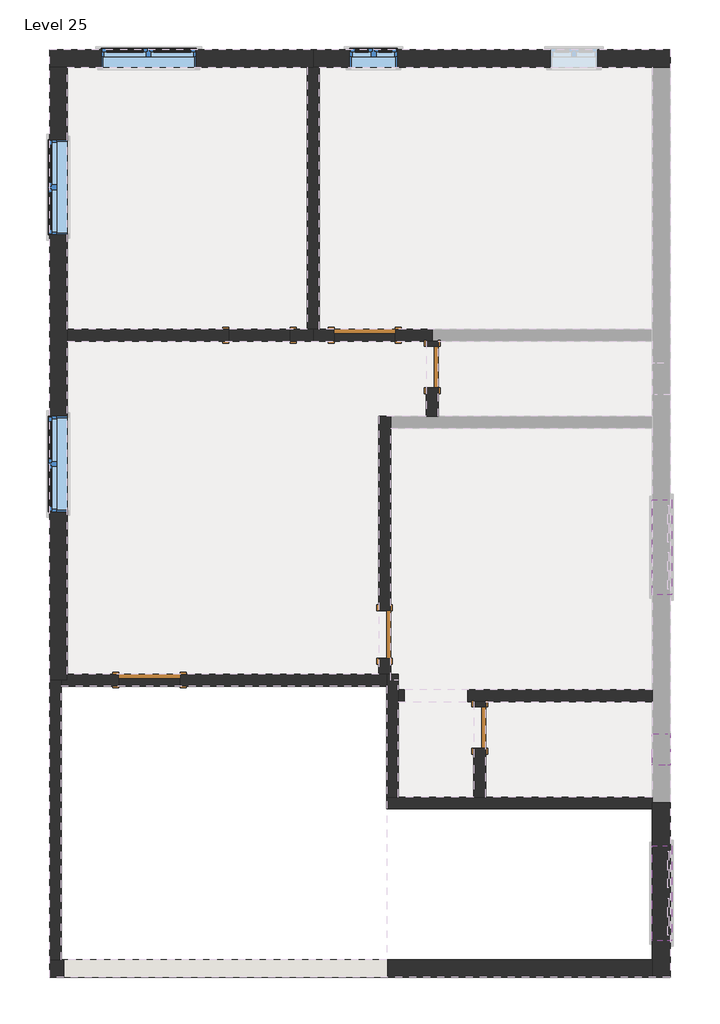
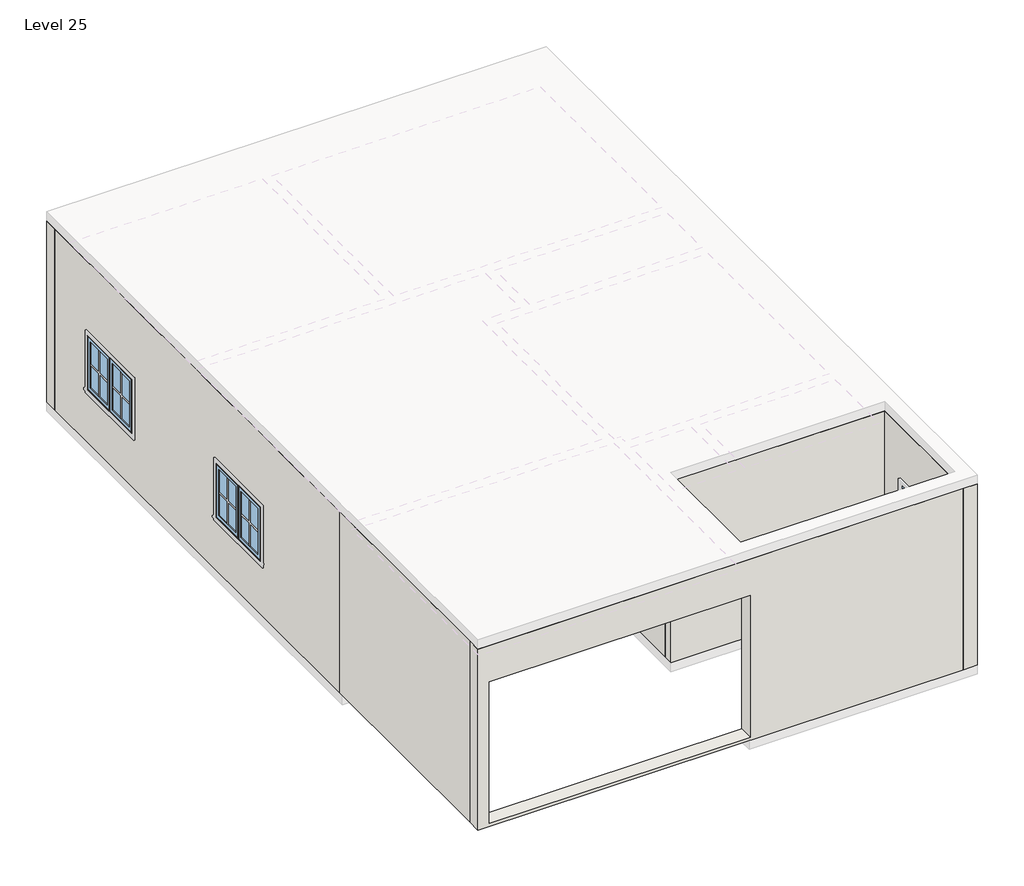
# One storey, part 1 of 2: 24 walls, 10 windows, 6 doors.
"""IFC4 building model written with IfcOpenShell, lengths in millimetres."""

from ifc_helpers import new_model, si_unit, frame, origin, place, context, project, spatial, polyline, outline, extrude, faceted_brep, transform, mapped, element, save
from components import door_2908be75, door_9ea4ff49, door_dc34e247, door_b804d09e, fixed_2_415b3208, window_casement_double_3_c417fced, window_casement_double_4_c19c33cb

model = new_model("IFC4")

# Units and contexts
model_context = context("Model", 3, world=origin())
ifc_project = project(units=[si_unit("LENGTHUNIT", "METRE", prefix="MILLI")], contexts=[model_context])

# Site, building, storey
site = spatial("IfcSite", under=ifc_project)
building = spatial("IfcBuilding", under=site)
storey = spatial("IfcBuildingStorey", under=building, Name="Level 25", Elevation=22402.8)

# Doors
placement = place(None, origin())
door_shape = door_2908be75(model_context)
element("IfcDoor", 1, ObjectType="Single-Flush : 1' 9\"", at=placement, inside=storey, context=model_context, shape_type="MappedRepresentation", body=[
    mapped(door_shape, transform((-397.3154463, -2781.5544725, 22402.8), x_axis=(0.0, 1.0, 0.0), y_axis=(-1.0, 0.0, 0.0), z_axis=(0.0, 0.0, 1.0))),
])
element("IfcDoor", 2, ObjectType="Single-Flush : 1' 9\"", at=placement, inside=storey, context=model_context, shape_type="MappedRepresentation", body=[
    mapped(door_shape, transform((-1006.9154463, 1841.2455275, 22402.8), x_axis=(0.0, 1.0, 0.0), y_axis=(-1.0, 0.0, 0.0), z_axis=(0.0, 0.0, 1.0))),
])
door_2_shape = door_9ea4ff49(model_context)
element("IfcDoor", 3, ObjectType="Single-Flush : 2'0\"", at=placement, inside=storey, context=model_context, shape_type="MappedRepresentation", body=[
    mapped(door_2_shape, transform((-1616.5154463, -1587.7544725, 22402.8), x_axis=(0.0, -1.0, 0.0), y_axis=(1.0, 0.0, 0.0), z_axis=(0.0, 0.0, 1.0))),
])
door_3_shape = door_dc34e247(model_context)
element("IfcDoor", 4, ObjectType="Single-Flush : 2'7\"", at=placement, inside=storey, context=model_context, shape_type="MappedRepresentation", body=[
    mapped(door_3_shape, transform((-4626.4154463, -2171.9544725, 22402.8), x_axis=(-1.0, 0.0, 0.0), y_axis=(0.0, -1.0, 0.0), z_axis=(0.0, 0.0, 1.0))),
])
element("IfcDoor", 5, ObjectType="Single-Flush : 2'7\"", at=placement, inside=storey, context=model_context, shape_type="MappedRepresentation", body=[
    mapped(door_3_shape, transform((-1870.5154463, 2247.6455275, 22402.8), x_axis=(-1.0, 0.0, 0.0), y_axis=(0.0, -1.0, 0.0), z_axis=(0.0, 0.0, 1.0))),
])
door_4_shape = door_b804d09e(model_context)
element("IfcDoor", 6, ObjectType="Single-Flush : 2'7\"", at=placement, inside=storey, context=model_context, shape_type="MappedRepresentation", body=[
    mapped(door_4_shape, transform((-3216.7154463, 2247.6455275, 22402.8), x_axis=(1.0, 0.0, 0.0), y_axis=(0.0, 1.0, 0.0), z_axis=(0.0, 0.0, 1.0))),
])

# Walls
element("IfcWall", 7, ObjectType="Generic - 6\"", at=placement, inside=storey, context=model_context, shape_type="Brep", body=[
    faceted_brep([(-5909.1154463, -2171.9544725, 22402.8), (-5909.1154463, -5753.3544725, 22402.8), (-5909.1154463, -5753.3544725, 25450.8), (-5909.1154463, -2171.9544725, 25450.8), (-5756.7154463, -2171.9544725, 22402.8), (-5756.7154463, -2171.9544725, 25450.8), (-5756.7154463, -2248.1544725, 25450.8), (-5756.7154463, -5753.3544725, 25450.8), (-5756.7154463, -5753.3544725, 22402.8), (-5756.7154463, -2248.1544725, 22402.8)], [[[0, 1, 2, 3]], [[4, 5, 6, 7, 8, 9]], [[1, 0, 4, 9, 8]], [[3, 2, 7, 6, 5]], [[0, 3, 5, 4]], [[2, 1, 8, 7]]]),
])
element("IfcWall", 8, ObjectType="Generic - 6\"", at=placement, inside=storey, context=model_context, shape_type="Brep", body=[
    faceted_brep([(1812.4845537, -3670.5544725, 22402.8), (-321.1154463, -3670.5544725, 22402.8), (-473.5154463, -3670.5544725, 22402.8), (-1438.7154463, -3670.5544725, 22402.8), (-1591.1154463, -3670.5544725, 22402.8), (-1591.1154463, -3670.5544725, 25450.8), (-1438.7154463, -3670.5544725, 25450.8), (-473.5154463, -3670.5544725, 25450.8), (-321.1154463, -3670.5544725, 25450.8), (1812.4845537, -3670.5544725, 25450.8), (1812.4845537, -3822.9544725, 22402.8), (1812.4845537, -3822.9544725, 25450.8), (-1591.1154463, -3822.9544725, 25450.8), (-1591.1154463, -3822.9544725, 22402.8), (1812.4845537, -3746.7544725, 22402.8), (1812.4845537, -3746.7544725, 25450.8)], [[[0, 1, 2, 3, 4, 5, 6, 7, 8, 9]], [[10, 11, 12, 13]], [[4, 3, 2, 1, 0, 14, 10, 13]], [[9, 8, 7, 6, 5, 12, 11, 15]], [[5, 4, 13, 12]], [[0, 9, 15, 11, 10, 14]]]),
])
element("IfcWall", 9, ObjectType="Generic - 6\"", at=placement, inside=storey, context=model_context, shape_type="Brep", body=[
    faceted_brep([(-1438.7154463, -3670.5544725, 22402.8), (-1438.7154463, -2451.3544725, 22402.8), (-1438.7154463, -2298.9544725, 22402.8), (-1438.7154463, -2095.7544725, 22402.8), (-1438.7154463, -2095.7544725, 25450.8), (-1438.7154463, -2298.9544725, 25450.8), (-1438.7154463, -2451.3544725, 25450.8), (-1438.7154463, -3670.5544725, 25450.8), (-1591.1154463, -3670.5544725, 22402.8), (-1591.1154463, -3670.5544725, 25450.8), (-1591.1154463, -2248.1544725, 25450.8), (-1591.1154463, -2171.9544725, 25450.8), (-1591.1154463, -2095.7544725, 25450.8), (-1591.1154463, -2095.7544725, 22402.8), (-1591.1154463, -2171.9544725, 22402.8), (-1591.1154463, -2248.1544725, 22402.8), (-1540.3154463, -2095.7544725, 22402.8), (-1540.3154463, -2095.7544725, 25450.8)], [[[0, 1, 2, 3, 4, 5, 6, 7]], [[8, 9, 10, 11, 12, 13, 14, 15]], [[3, 2, 1, 0, 8, 15, 14, 13, 16]], [[7, 6, 5, 4, 17, 12, 11, 10, 9]], [[0, 7, 9, 8]], [[4, 3, 16, 13, 12, 17]]]),
])
element("IfcWall", 10, ObjectType="Generic - 6\"", at=placement, inside=storey, context=model_context, shape_type="Brep", body=[
    faceted_brep([(-5020.1154463, -2095.7544725, 24536.4), (-5020.1154463, -2095.7544725, 22402.8), (-5680.5154463, -2095.7544725, 22402.8), (-5680.5154463, -2095.7544725, 25450.8), (-1692.7154463, -2095.7544725, 25450.8), (-1591.1154463, -2095.7544725, 25450.8), (-1591.1154463, -2095.7544725, 22402.8), (-1692.7154463, -2095.7544725, 22402.8), (-4232.7154463, -2095.7544725, 22402.8), (-4232.7154463, -2095.7544725, 24536.4), (-5756.7154463, -2248.1544725, 22402.8), (-5020.1154463, -2248.1544725, 22402.8), (-5020.1154463, -2248.1544725, 24536.4), (-4232.7154463, -2248.1544725, 24536.4), (-4232.7154463, -2248.1544725, 22402.8), (-1591.1154463, -2248.1544725, 22402.8), (-1591.1154463, -2248.1544725, 25450.8), (-5756.7154463, -2248.1544725, 25450.8), (-5756.7154463, -2171.9544725, 22402.8), (-5680.5154463, -2171.9544725, 22402.8), (-5680.5154463, -2171.9544725, 25450.8), (-5756.7154463, -2171.9544725, 25450.8)], [[[0, 1, 2, 3, 4, 5, 6, 7, 8, 9]], [[10, 11, 12, 13, 14, 15, 16, 17]], [[2, 1, 11, 10, 18, 19]], [[8, 7, 6, 15, 14]], [[5, 4, 3, 20, 21, 17, 16]], [[3, 2, 19, 20]], [[19, 18, 21, 20]], [[18, 10, 17, 21]], [[6, 5, 16, 15]], [[12, 11, 1, 0]], [[13, 12, 0, 9]], [[14, 13, 9, 8]]]),
])
element("IfcWall", 11, ObjectType="Generic - 6\"", at=placement, inside=storey, context=model_context, shape_type="Brep", body=[
    faceted_brep([(1812.4845537, -2451.3544725, 22402.8), (1812.4845537, -2451.3544725, 25450.8), (-321.1154463, -2451.3544725, 25450.8), (-473.5154463, -2451.3544725, 25450.8), (-1438.7154463, -2451.3544725, 25450.8), (-1438.7154463, -2451.3544725, 22402.8), (-1367.0206652, -2451.3544725, 22402.8), (-1367.0206652, -2451.3544725, 24841.2), (-547.4818767, -2451.3544725, 24841.2), (-547.4818767, -2451.3544725, 22402.8), (-473.5154463, -2451.3544725, 22402.8), (-321.1154463, -2451.3544725, 22402.8), (1812.4845537, -2298.9544725, 25450.8), (1812.4845537, -2298.9544725, 22402.8), (-547.4818767, -2298.9544725, 22402.8), (-547.4818767, -2298.9544725, 24841.2), (-1367.0206652, -2298.9544725, 24841.2), (-1367.0206652, -2298.9544725, 22402.8), (-1438.7154463, -2298.9544725, 22402.8), (-1438.7154463, -2298.9544725, 25450.8)], [[[0, 1, 2, 3, 4, 5, 6, 7, 8, 9, 10, 11]], [[12, 13, 14, 15, 16, 17, 18, 19]], [[5, 18, 17, 6]], [[13, 0, 11, 10, 9, 14]], [[4, 3, 2, 1, 12, 19]], [[1, 0, 13, 12]], [[5, 4, 19, 18]], [[7, 16, 15, 8]], [[16, 7, 6, 17]], [[8, 15, 14, 9]]]),
])
element("IfcWall", 12, ObjectType="Generic - 6\"", at=placement, inside=storey, context=model_context, shape_type="SweptSolid", body=[
    extrude(outline(polyline([(-2451.3544725, 22402.8), (-2514.8544725, 22402.8), (-2514.8544725, 24536.4), (-3048.2544725, 24536.4), (-3048.2544725, 22402.8), (-3670.5544725, 22402.8), (-3670.5544725, 25450.8), (-2451.3544725, 25450.8), (-2451.3544725, 22402.8)])), frame((-473.5154463, 0.0, 0.0), z_axis=(1.0, 0.0, 0.0), x_axis=(0.0, 1.0, 0.0)), (0.0, 0.0, 1.0), 152.4),
])
element("IfcWall", 13, ObjectType="Generic - 6\"", at=placement, inside=storey, context=model_context, shape_type="Brep", body=[
    faceted_brep([(-1540.3154463, -2095.7544725, 22402.8), (-1540.3154463, -1892.5544725, 22402.8), (-1540.3154463, -1892.5544725, 24536.4), (-1540.3154463, -1282.9544725, 24536.4), (-1540.3154463, -1282.9544725, 22402.8), (-1540.3154463, 1053.8455275, 22402.8), (-1540.3154463, 1206.2455275, 22402.8), (-1540.3154463, 1206.2455275, 25450.8), (-1540.3154463, 1053.8455275, 25450.8), (-1540.3154463, -2095.7544725, 25450.8), (-1692.7154463, -1892.5544725, 24536.4), (-1692.7154463, -1892.5544725, 22402.8), (-1692.7154463, -2095.7544725, 22402.8), (-1692.7154463, -2095.7544725, 25450.8), (-1692.7154463, 1206.2455275, 25450.8), (-1692.7154463, 1206.2455275, 22402.8), (-1692.7154463, -1282.9544725, 22402.8), (-1692.7154463, -1282.9544725, 24536.4), (-1591.1154463, -2095.7544725, 22402.8), (-1591.1154463, -2095.7544725, 25450.8)], [[[0, 1, 2, 3, 4, 5, 6, 7, 8, 9]], [[10, 11, 12, 13, 14, 15, 16, 17]], [[16, 15, 6, 5, 4]], [[12, 11, 1, 0, 18]], [[9, 8, 7, 14, 13, 19]], [[0, 9, 19, 13, 12, 18]], [[7, 6, 15, 14]], [[2, 1, 11, 10]], [[3, 2, 10, 17]], [[4, 3, 17, 16]]]),
])
element("IfcWall", 14, ObjectType="Generic - 6\"", at=placement, inside=storey, context=model_context, shape_type="Brep", body=[
    faceted_brep([(-930.7154463, 2107.9455275, 24536.4), (-930.7154463, 2107.9455275, 22402.8), (-930.7154463, 2171.4455275, 22402.8), (-930.7154463, 2171.4455275, 25450.8), (-930.7154463, 1206.2455275, 25450.8), (-930.7154463, 1206.2455275, 22402.8), (-930.7154463, 1574.5455275, 22402.8), (-930.7154463, 1574.5455275, 24536.4), (-1083.1154463, 2171.4455275, 22402.8), (-1083.1154463, 2107.9455275, 22402.8), (-1083.1154463, 2107.9455275, 24536.4), (-1083.1154463, 1574.5455275, 24536.4), (-1083.1154463, 1574.5455275, 22402.8), (-1083.1154463, 1206.2455275, 22402.8), (-1083.1154463, 1206.2455275, 25450.8), (-1083.1154463, 2171.4455275, 25450.8), (-1006.9154463, 2171.4455275, 22402.8), (-1006.9154463, 2171.4455275, 25450.8)], [[[0, 1, 2, 3, 4, 5, 6, 7]], [[8, 9, 10, 11, 12, 13, 14, 15]], [[6, 5, 13, 12]], [[2, 1, 9, 8, 16]], [[4, 3, 17, 15, 14]], [[5, 4, 14, 13]], [[10, 9, 1, 0]], [[11, 10, 0, 7]], [[12, 11, 7, 6]], [[3, 2, 16, 8, 15, 17]]]),
])
element("IfcWall", 15, ObjectType="Generic - 6\"", at=placement, inside=storey, context=model_context, shape_type="Brep", body=[
    faceted_brep([(-2607.1154463, 5678.2330275, 22402.8), (-2607.1154463, 2323.8455275, 22402.8), (-2607.1154463, 2323.8455275, 25450.8), (-2607.1154463, 5678.2330275, 25450.8), (-2454.7154463, 5678.2330275, 22402.8), (-2454.7154463, 5678.2330275, 25450.8), (-2454.7154463, 2323.8455275, 25450.8), (-2454.7154463, 2323.8455275, 22402.8), (-2530.9154463, 5678.2330275, 22402.8), (-2530.9154463, 2323.8455275, 22402.8), (-2530.9154463, 2323.8455275, 25450.8), (-2530.9154463, 5678.2330275, 25450.8)], [[[0, 1, 2, 3]], [[4, 5, 6, 7]], [[1, 0, 8, 4, 7, 9]], [[3, 2, 10, 6, 5, 11]], [[0, 3, 11, 5, 4, 8]], [[2, 1, 9, 7, 6, 10]]]),
])
element("IfcWall", 16, ObjectType="Generic - 6\"", at=placement, inside=storey, context=model_context, shape_type="Brep", body=[
    faceted_brep([(-2530.9154463, 2323.8455275, 22402.8), (-2607.1154463, 2323.8455275, 22402.8), (-2823.0154463, 2323.8455275, 22402.8), (-2823.0154463, 2323.8455275, 24536.4), (-3610.4154463, 2323.8455275, 24536.4), (-3610.4154463, 2323.8455275, 22402.8), (-5680.5154463, 2323.8455275, 22402.8), (-5680.5154463, 2323.8455275, 25450.8), (-2607.1154463, 2323.8455275, 25450.8), (-2530.9154463, 2323.8455275, 25450.8), (-2823.0154463, 2171.4455275, 24536.4), (-2823.0154463, 2171.4455275, 22402.8), (-2530.9154463, 2171.4455275, 22402.8), (-2530.9154463, 2171.4455275, 25450.8), (-5680.5154463, 2171.4455275, 25450.8), (-5680.5154463, 2171.4455275, 22402.8), (-3610.4154463, 2171.4455275, 22402.8), (-3610.4154463, 2171.4455275, 24536.4)], [[[0, 1, 2, 3, 4, 5, 6, 7, 8, 9]], [[10, 11, 12, 13, 14, 15, 16, 17]], [[16, 15, 6, 5]], [[12, 11, 2, 1, 0]], [[9, 8, 7, 14, 13]], [[0, 9, 13, 12]], [[7, 6, 15, 14]], [[5, 4, 17, 16]], [[4, 3, 10, 17]], [[3, 2, 11, 10]]]),
])
element("IfcWall", 17, ObjectType="Generic - 6\"", at=placement, inside=storey, context=model_context, shape_type="Brep", body=[
    faceted_brep([(-2264.2154463, 2323.8455275, 24536.4), (-2264.2154463, 2323.8455275, 22402.8), (-2454.7154463, 2323.8455275, 22402.8), (-2530.9154463, 2323.8455275, 22402.8), (-2530.9154463, 2323.8455275, 25450.8), (-2454.7154463, 2323.8455275, 25450.8), (-1006.9154463, 2323.8455275, 25450.8), (-1006.9154463, 2323.8455275, 22402.8), (-1476.8154463, 2323.8455275, 22402.8), (-1476.8154463, 2323.8455275, 24536.4), (-2530.9154463, 2171.4455275, 22402.8), (-2264.2154463, 2171.4455275, 22402.8), (-2264.2154463, 2171.4455275, 24536.4), (-1476.8154463, 2171.4455275, 24536.4), (-1476.8154463, 2171.4455275, 22402.8), (-1083.1154463, 2171.4455275, 22402.8), (-1006.9154463, 2171.4455275, 22402.8), (-1006.9154463, 2171.4455275, 25450.8), (-1083.1154463, 2171.4455275, 25450.8), (-2530.9154463, 2171.4455275, 25450.8)], [[[0, 1, 2, 3, 4, 5, 6, 7, 8, 9]], [[10, 11, 12, 13, 14, 15, 16, 17, 18, 19]], [[8, 7, 16, 15, 14]], [[3, 2, 1, 11, 10]], [[4, 3, 10, 19]], [[6, 5, 4, 19, 18, 17]], [[7, 6, 17, 16]], [[14, 13, 9, 8]], [[13, 12, 0, 9]], [[12, 11, 1, 0]]]),
])
element("IfcWall", 18, ObjectType="Generic - 6\"", at=placement, inside=storey, context=model_context, shape_type="SweptSolid", body=[
    extrude(outline(polyline([(-5680.5154463, -2095.7544725), (-1692.7154463, -2095.7544725), (-1692.7154463, -2171.9544725), (-1591.1154463, -2171.9544725), (-1591.1154463, -2248.1544725), (-5756.7154463, -2248.1544725), (-5756.7154463, -2171.9544725), (-5680.5154463, -2171.9544725), (-5680.5154463, -2095.7544725)])), frame((0.0, 0.0, 22402.8), z_axis=(0.0, 0.0, 1.0), x_axis=(1.0, 0.0, 0.0)), (0.0, 0.0, 1.0), 3048.0),
])
element("IfcWall", 19, ObjectType="Generic - 6\"", at=placement, inside=storey, context=model_context, shape_type="Brep", body=[
    faceted_brep([(-2607.1154463, 5678.2330275, 22402.8), (-2607.1154463, 2323.8455275, 22402.8), (-2607.1154463, 2323.8455275, 25450.8), (-2607.1154463, 5678.2330275, 25450.8), (-2454.7154463, 5678.2330275, 22402.8), (-2454.7154463, 5678.2330275, 25450.8), (-2454.7154463, 2323.8455275, 25450.8), (-2454.7154463, 2323.8455275, 22402.8), (-2530.9154463, 5678.2330275, 22402.8), (-2530.9154463, 2323.8455275, 22402.8), (-2530.9154463, 2323.8455275, 25450.8), (-2530.9154463, 5678.2330275, 25450.8)], [[[0, 1, 2, 3]], [[4, 5, 6, 7]], [[1, 0, 8, 4, 7, 9]], [[3, 2, 10, 6, 5, 11]], [[0, 3, 11, 5, 4, 8]], [[2, 1, 9, 7, 6, 10]]]),
])
element("IfcWall", 20, ObjectType="Generic - 6\"", at=placement, inside=storey, context=model_context, shape_type="Brep", body=[
    faceted_brep([(-2530.9154463, 2323.8455275, 22402.8), (-2607.1154463, 2323.8455275, 22402.8), (-5680.5154463, 2323.8455275, 22402.8), (-5680.5154463, 2323.8455275, 25450.8), (-2607.1154463, 2323.8455275, 25450.8), (-2530.9154463, 2323.8455275, 25450.8), (-2530.9154463, 2171.4455275, 22402.8), (-2530.9154463, 2171.4455275, 25450.8), (-5680.5154463, 2171.4455275, 25450.8), (-5680.5154463, 2171.4455275, 22402.8)], [[[0, 1, 2, 3, 4, 5]], [[6, 7, 8, 9]], [[2, 1, 0, 6, 9]], [[5, 4, 3, 8, 7]], [[0, 5, 7, 6]], [[3, 2, 9, 8]]]),
])
element("IfcWall", 21, ObjectType="Generic - 6\"", at=placement, inside=storey, context=model_context, shape_type="Brep", body=[
    faceted_brep([(-1006.9154463, 2323.8455275, 22402.8), (-2454.7154463, 2323.8455275, 22402.8), (-2530.9154463, 2323.8455275, 22402.8), (-2530.9154463, 2323.8455275, 25450.8), (-2454.7154463, 2323.8455275, 25450.8), (-1006.9154463, 2323.8455275, 25450.8), (-1006.9154463, 2171.4455275, 22402.8), (-1006.9154463, 2171.4455275, 25450.8), (-1083.1154463, 2171.4455275, 25450.8), (-2530.9154463, 2171.4455275, 25450.8), (-2530.9154463, 2171.4455275, 22402.8), (-1083.1154463, 2171.4455275, 22402.8)], [[[0, 1, 2, 3, 4, 5]], [[6, 7, 8, 9, 10, 11]], [[2, 1, 0, 6, 11, 10]], [[3, 2, 10, 9]], [[5, 4, 3, 9, 8, 7]], [[0, 5, 7, 6]]]),
])
element("IfcWall", 22, ObjectType="Generic - 9\"", at=placement, inside=storey, context=model_context, shape_type="Brep", body=[
    faceted_brep([(-5909.1154463, 5678.2330275, 22402.8), (-5680.5154463, 5678.2330275, 22402.8), (-2607.1154463, 5678.2330275, 22402.8), (-2530.9154463, 5678.2330275, 22402.8), (-2530.9154463, 5678.2330275, 25450.8), (-2607.1154463, 5678.2330275, 25450.8), (-5680.5154463, 5678.2330275, 25450.8), (-5909.1154463, 5678.2330275, 25450.8), (-4029.5154463, 5678.2330275, 24231.6), (-4029.5154463, 5678.2330275, 23317.2), (-5248.7154463, 5678.2330275, 23317.2), (-5248.7154463, 5678.2330275, 24231.6), (-5909.1154463, 5906.8330275, 22402.8), (-5909.1154463, 5906.8330275, 25450.8), (-2530.9154463, 5906.8330275, 25450.8), (-2530.9154463, 5906.8330275, 22402.8), (-4029.5154463, 5906.8330275, 24231.6), (-5248.7154463, 5906.8330275, 24231.6), (-5248.7154463, 5906.8330275, 23317.2), (-4029.5154463, 5906.8330275, 23317.2)], [[[0, 1, 2, 3, 4, 5, 6, 7], [8, 9, 10, 11]], [[12, 13, 14, 15], [16, 17, 18, 19]], [[3, 2, 1, 0, 12, 15]], [[4, 3, 15, 14]], [[7, 6, 5, 4, 14, 13]], [[0, 7, 13, 12]], [[9, 8, 16, 19]], [[10, 9, 19, 18]], [[11, 10, 18, 17]], [[8, 11, 17, 16]]]),
])
element("IfcWall", 23, ObjectType="Generic - 9\"", at=placement, inside=storey, context=model_context, shape_type="Brep", body=[
    faceted_brep([(1812.4845537, -5753.3544725, 22402.8), (-5756.7154463, -5753.3544725, 22402.8), (-5909.1154463, -5753.3544725, 22402.8), (-5909.1154463, -5753.3544725, 25450.8), (-5756.7154463, -5753.3544725, 25450.8), (1812.4845537, -5753.3544725, 25450.8), (-1576.8982041, -5753.3544725, 24841.2), (-5729.1673724, -5753.3544725, 24841.2), (-5729.1673724, -5753.3544725, 22453.6), (-1576.8982041, -5753.3544725, 22453.6), (-5909.1154463, -5981.9544725, 22402.8), (1812.4845537, -5981.9544725, 22402.8), (1812.4845537, -5981.9544725, 25450.8), (-5909.1154463, -5981.9544725, 25450.8), (-5729.1673724, -5981.9544725, 24841.2), (-1576.8982041, -5981.9544725, 24841.2), (-1576.8982041, -5981.9544725, 22453.6), (-5729.1673724, -5981.9544725, 22453.6)], [[[0, 1, 2, 3, 4, 5], [6, 7, 8, 9]], [[10, 11, 12, 13], [14, 15, 16, 17]], [[2, 1, 0, 11, 10]], [[5, 4, 3, 13, 12]], [[0, 5, 12, 11]], [[6, 15, 14, 7]], [[8, 17, 16, 9]], [[15, 6, 9, 16]], [[7, 14, 17, 8]], [[3, 2, 10, 13]]]),
])
element("IfcWall", 24, ObjectType="Generic - 9\"", at=placement, inside=storey, context=model_context, shape_type="Brep", body=[
    faceted_brep([(-5909.1154463, 5678.2330275, 22402.8), (-5909.1154463, -2171.9544725, 22402.8), (-5909.1154463, -2171.9544725, 25450.8), (-5909.1154463, 5678.2330275, 25450.8), (-5909.1154463, 4751.1330275, 24231.6), (-5909.1154463, 3531.9330275, 24231.6), (-5909.1154463, 3531.9330275, 23317.2), (-5909.1154463, 4751.1330275, 23317.2), (-5909.1154463, 1206.2455275, 24231.6), (-5909.1154463, -12.9544725, 24231.6), (-5909.1154463, -12.9544725, 23317.2), (-5909.1154463, 1206.2455275, 23317.2), (-5680.5154463, 5678.2330275, 22402.8), (-5680.5154463, 5678.2330275, 25450.8), (-5680.5154463, 2323.8455275, 25450.8), (-5680.5154463, 2171.4455275, 25450.8), (-5680.5154463, -2095.7544725, 25450.8), (-5680.5154463, -2171.9544725, 25450.8), (-5680.5154463, -2171.9544725, 22402.8), (-5680.5154463, -2095.7544725, 22402.8), (-5680.5154463, 2171.4455275, 22402.8), (-5680.5154463, 2323.8455275, 22402.8), (-5680.5154463, 4751.1330275, 24231.6), (-5680.5154463, 4751.1330275, 23317.2), (-5680.5154463, 3531.9330275, 23317.2), (-5680.5154463, 3531.9330275, 24231.6), (-5680.5154463, 1206.2455275, 24231.6), (-5680.5154463, 1206.2455275, 23317.2), (-5680.5154463, -12.9544725, 23317.2), (-5680.5154463, -12.9544725, 24231.6), (-5756.7154463, -2171.9544725, 22402.8), (-5756.7154463, -2171.9544725, 25450.8)], [[[0, 1, 2, 3], [4, 5, 6, 7], [8, 9, 10, 11]], [[12, 13, 14, 15, 16, 17, 18, 19, 20, 21], [22, 23, 24, 25], [26, 27, 28, 29]], [[1, 0, 12, 21, 20, 19, 18, 30]], [[2, 1, 30, 18, 17, 31]], [[3, 2, 31, 17, 16, 15, 14, 13]], [[0, 3, 13, 12]], [[23, 22, 4, 7]], [[24, 23, 7, 6]], [[25, 24, 6, 5]], [[22, 25, 5, 4]], [[27, 26, 8, 11]], [[28, 27, 11, 10]], [[29, 28, 10, 9]], [[26, 29, 9, 8]]]),
])
element("IfcWall", 25, ObjectType="Generic - 9\"", at=placement, inside=storey, context=model_context, shape_type="Brep", body=[
    faceted_brep([(-2530.9154463, 5678.2330275, 22402.8), (-2454.7154463, 5678.2330275, 22402.8), (1812.4845537, 5678.2330275, 22402.8), (2041.0845537, 5678.2330275, 22402.8), (2041.0845537, 5678.2330275, 25450.8), (1812.4845537, 5678.2330275, 25450.8), (-2454.7154463, 5678.2330275, 25450.8), (-2530.9154463, 5678.2330275, 25450.8), (-1451.4154463, 5678.2330275, 24231.6), (-1451.4154463, 5678.2330275, 23317.2), (-2061.0154463, 5678.2330275, 23317.2), (-2061.0154463, 5678.2330275, 24231.6), (1113.9845537, 5678.2330275, 24231.6), (1113.9845537, 5678.2330275, 23317.2), (504.3845537, 5678.2330275, 23317.2), (504.3845537, 5678.2330275, 24231.6), (-2530.9154463, 5906.8330275, 22402.8), (-2530.9154463, 5906.8330275, 25450.8), (2041.0845537, 5906.8330275, 25450.8), (2041.0845537, 5906.8330275, 22402.8), (-1451.4154463, 5906.8330275, 24231.6), (-2061.0154463, 5906.8330275, 24231.6), (-2061.0154463, 5906.8330275, 23317.2), (-1451.4154463, 5906.8330275, 23317.2), (1113.9845537, 5906.8330275, 24231.6), (504.3845537, 5906.8330275, 24231.6), (504.3845537, 5906.8330275, 23317.2), (1113.9845537, 5906.8330275, 23317.2)], [[[0, 1, 2, 3, 4, 5, 6, 7], [8, 9, 10, 11], [12, 13, 14, 15]], [[16, 17, 18, 19], [20, 21, 22, 23], [24, 25, 26, 27]], [[3, 2, 1, 0, 16, 19]], [[7, 6, 5, 4, 18, 17]], [[0, 7, 17, 16]], [[4, 3, 19, 18]], [[8, 11, 21, 20]], [[11, 10, 22, 21]], [[10, 9, 23, 22]], [[9, 8, 20, 23]], [[12, 15, 25, 24]], [[15, 14, 26, 25]], [[14, 13, 27, 26]], [[13, 12, 24, 27]]]),
])
element("IfcWall", 26, ObjectType="Generic - 9\"", at=placement, inside=storey, context=model_context, shape_type="Brep", body=[
    faceted_brep([(1812.4845537, -3746.7544725, 22402.8), (1812.4845537, -3822.9544725, 22402.8), (1812.4845537, -5753.3544725, 22402.8), (1812.4845537, -5981.9544725, 22402.8), (1812.4845537, -5981.9544725, 25450.8), (1812.4845537, -5753.3544725, 25450.8), (1812.4845537, -3822.9544725, 25450.8), (1812.4845537, -3746.7544725, 25450.8), (1812.4845537, -5512.0544725, 24536.4), (1812.4845537, -5512.0544725, 23622.0), (1812.4845537, -4292.8544725, 23622.0), (1812.4845537, -4292.8544725, 24536.4), (2041.0845537, -3746.7544725, 22402.8), (2041.0845537, -3746.7544725, 25450.8), (2041.0845537, -5981.9544725, 25450.8), (2041.0845537, -5981.9544725, 22402.8), (2041.0845537, -5512.0544725, 24536.4), (2041.0845537, -4292.8544725, 24536.4), (2041.0845537, -4292.8544725, 23622.0), (2041.0845537, -5512.0544725, 23622.0)], [[[0, 1, 2, 3, 4, 5, 6, 7], [8, 9, 10, 11]], [[12, 13, 14, 15], [16, 17, 18, 19]], [[3, 2, 1, 0, 12, 15]], [[7, 6, 5, 4, 14, 13]], [[0, 7, 13, 12]], [[4, 3, 15, 14]], [[8, 11, 17, 16]], [[11, 10, 18, 17]], [[10, 9, 19, 18]], [[9, 8, 16, 19]]]),
])
element("IfcWall", 27, ObjectType="Generic - 9\"", at=placement, inside=storey, context=model_context, shape_type="SweptSolid", body=[
    extrude(outline(polyline([(22402.8, -5680.5154463), (22402.8, -2607.1154463), (25450.8, -2607.1154463), (25450.8, -5680.5154463), (22402.8, -5680.5154463)]), holes=[polyline([(24231.6, -4029.5154463), (23317.2, -4029.5154463), (23317.2, -5248.7154463), (24231.6, -5248.7154463), (24231.6, -4029.5154463)])]), frame((0.0, 5678.2330275, 0.0), z_axis=(0.0, 1.0, 0.0), x_axis=(0.0, 0.0, 1.0)), (0.0, 0.0, 1.0), 228.6),
])
element("IfcWall", 28, ObjectType="Generic - 9\"", at=placement, inside=storey, context=model_context, shape_type="Brep", body=[
    faceted_brep([(1812.4845537, -5753.3544725, 22402.8), (-5756.7154463, -5753.3544725, 22402.8), (-5909.1154463, -5753.3544725, 22402.8), (-5909.1154463, -5753.3544725, 25450.8), (-5756.7154463, -5753.3544725, 25450.8), (1812.4845537, -5753.3544725, 25450.8), (-1576.8982041, -5753.3544725, 24841.2), (-5729.1673724, -5753.3544725, 24841.2), (-5729.1673724, -5753.3544725, 22453.6), (-1576.8982041, -5753.3544725, 22453.6), (-5909.1154463, -5981.9544725, 22402.8), (1812.4845537, -5981.9544725, 22402.8), (1812.4845537, -5981.9544725, 25450.8), (-5909.1154463, -5981.9544725, 25450.8), (-5729.1673724, -5981.9544725, 24841.2), (-1576.8982041, -5981.9544725, 24841.2), (-1576.8982041, -5981.9544725, 22453.6), (-5729.1673724, -5981.9544725, 22453.6)], [[[0, 1, 2, 3, 4, 5], [6, 7, 8, 9]], [[10, 11, 12, 13], [14, 15, 16, 17]], [[2, 1, 0, 11, 10]], [[5, 4, 3, 13, 12]], [[6, 15, 14, 7]], [[8, 17, 16, 9]], [[15, 6, 9, 16]], [[7, 14, 17, 8]], [[3, 2, 10, 13]], [[0, 5, 12, 11]]]),
])
element("IfcWall", 29, ObjectType="Generic - 9\"", at=placement, inside=storey, context=model_context, shape_type="SweptSolid", body=[
    extrude(outline(polyline([(22402.8, -2454.7154463), (22402.8, 1812.4845537), (25450.8, 1812.4845537), (25450.8, -2454.7154463), (22402.8, -2454.7154463)]), holes=[polyline([(24231.6, -1451.4154463), (23317.2, -1451.4154463), (23317.2, -2061.0154463), (24231.6, -2061.0154463), (24231.6, -1451.4154463)]), polyline([(24231.6, 1113.9845537), (23317.2, 1113.9845537), (23317.2, 504.3845537), (24231.6, 504.3845537), (24231.6, 1113.9845537)])]), frame((0.0, 5678.2330275, 0.0), z_axis=(0.0, 1.0, 0.0), x_axis=(0.0, 0.0, 1.0)), (0.0, 0.0, 1.0), 228.6),
])
element("IfcWall", 30, ObjectType="Generic - 9\"", at=placement, inside=storey, context=model_context, shape_type="SweptSolid", body=[
    extrude(outline(polyline([(-3822.9544725, 22402.8), (-5753.3544725, 22402.8), (-5753.3544725, 25450.8), (-3822.9544725, 25450.8), (-3822.9544725, 22402.8)]), holes=[polyline([(-5512.0544725, 24536.4), (-5512.0544725, 23622.0), (-4292.8544725, 23622.0), (-4292.8544725, 24536.4), (-5512.0544725, 24536.4)])]), frame((1812.4845537, 0.0, 0.0), z_axis=(1.0, 0.0, 0.0), x_axis=(0.0, 1.0, 0.0)), (0.0, 0.0, 1.0), 228.6),
])

# Windows
fixed_2_shape = fixed_2_415b3208(model_context)
element("IfcWindow", 31, ObjectType="Fixed : 2'", at=placement, inside=storey, context=model_context, shape_type="MappedRepresentation", body=[
    mapped(fixed_2_shape, transform((1926.7845537, -3099.0544725, 23926.8), x_axis=(0.0, -1.0, 0.0), y_axis=(1.0, 0.0, 0.0), z_axis=(0.0, 0.0, 1.0))),
])
window_casement_double_3_shape = window_casement_double_3_c417fced(model_context)
element("IfcWindow", 32, ObjectType="Window-Casement-Double : 3'", at=placement, inside=storey, context=model_context, shape_type="MappedRepresentation", body=[
    mapped(window_casement_double_3_shape, transform((-1756.2154463, 5792.5330275, 22402.8), x_axis=(1.0, 0.0, 0.0), y_axis=(0.0, 1.0, 0.0), z_axis=(0.0, 0.0, 1.0))),
])
element("IfcWindow", 33, ObjectType="Window-Casement-Double : 3'", at=placement, inside=storey, context=model_context, shape_type="MappedRepresentation", body=[
    mapped(window_casement_double_3_shape, transform((-1756.2154463, 5792.5330275, 22402.8), x_axis=(1.0, 0.0, 0.0), y_axis=(0.0, 1.0, 0.0), z_axis=(0.0, 0.0, 1.0))),
])
window_casement_double_4_shape = window_casement_double_4_c19c33cb(model_context)
element("IfcWindow", 34, ObjectType="Window-Casement-Double : 4'", at=placement, inside=storey, context=model_context, shape_type="MappedRepresentation", body=[
    mapped(window_casement_double_4_shape, transform((-4639.1154463, 5792.5330275, 22402.8), x_axis=(1.0, 0.0, 0.0), y_axis=(0.0, 1.0, 0.0), z_axis=(0.0, 0.0, 1.0))),
])
element("IfcWindow", 35, ObjectType="Window-Casement-Double : 4'", at=placement, inside=storey, context=model_context, shape_type="MappedRepresentation", body=[
    mapped(window_casement_double_4_shape, transform((-5794.8154463, 4141.5330275, 22402.8), x_axis=(0.0, 1.0, 0.0), y_axis=(-1.0, 0.0, 0.0), z_axis=(0.0, 0.0, 1.0))),
])
element("IfcWindow", 36, ObjectType="Window-Casement-Double : 4'", at=placement, inside=storey, context=model_context, shape_type="MappedRepresentation", body=[
    mapped(window_casement_double_4_shape, transform((-5794.8154463, 596.6455275, 22402.8), x_axis=(0.0, 1.0, 0.0), y_axis=(-1.0, 0.0, 0.0), z_axis=(0.0, 0.0, 1.0))),
])
element("IfcWindow", 37, ObjectType="Window-Casement-Double : 4'", at=placement, inside=storey, context=model_context, shape_type="MappedRepresentation", body=[
    mapped(window_casement_double_4_shape, transform((1926.7845537, -470.1544725, 22707.6), x_axis=(0.0, -1.0, 0.0), y_axis=(1.0, 0.0, 0.0), z_axis=(0.0, 0.0, 1.0))),
])
element("IfcWindow", 38, ObjectType="Window-Casement-Double : 4'", at=placement, inside=storey, context=model_context, shape_type="MappedRepresentation", body=[
    mapped(window_casement_double_4_shape, transform((1926.7845537, -4902.4544725, 22707.6), x_axis=(0.0, -1.0, 0.0), y_axis=(1.0, 0.0, 0.0), z_axis=(0.0, 0.0, 1.0))),
])
element("IfcWindow", 39, ObjectType="Window-Casement-Double : 4'", at=placement, inside=storey, context=model_context, shape_type="MappedRepresentation", body=[
    mapped(window_casement_double_4_shape, transform((-4639.1154463, 5792.5330275, 22402.8), x_axis=(1.0, 0.0, 0.0), y_axis=(0.0, 1.0, 0.0), z_axis=(0.0, 0.0, 1.0))),
])
element("IfcWindow", 40, ObjectType="Window-Casement-Double : 4'", at=placement, inside=storey, context=model_context, shape_type="MappedRepresentation", body=[
    mapped(window_casement_double_4_shape, transform((1926.7845537, -4902.4544725, 22707.6), x_axis=(0.0, -1.0, 0.0), y_axis=(1.0, 0.0, 0.0), z_axis=(0.0, 0.0, 1.0))),
])

save(model, "model.ifc")

# Revit data of these elements
# Type "Single-Flush : 1' 9\""
#   Type Mark = "10"
#   Construction Type Id = "MDOOR"
#   Assembly Code = "C1020"
#   Analytic Construction = "Metal"
#   Thickness = 0' - 2"
#   Heat Transfer Coefficient (U) = 0.651978 BTU/(h·ft²·°F)
#   Height = 7' - 0"
#   Trim Projection Ext = 0' - 1"
#   Trim Projection Int = 0' - 1"
#   Trim Width = 0' - 3"
#   Width = 1' - 9"
#   Define Thermal Properties by = 1
#   Door Material = Door - Panel
#   Frame Material = Door - Frame
#   Visual Light Transmittance = 0
#   Solar Heat Gain Coefficient = 0
#   Function = (empty or 0)
#   Wall Closure = (empty or 0)
# Type "Single-Flush : 2'0\""
#   Type Mark = "9"
#   Construction Type Id = "MDOOR"
#   Assembly Code = "C1020"
#   Analytic Construction = "Metal"
#   Thickness = 0' - 2"
#   Heat Transfer Coefficient (U) = 0.651978 BTU/(h·ft²·°F)
#   Height = 7' - 0"
#   Trim Projection Ext = 0' - 1"
#   Trim Projection Int = 0' - 1"
#   Trim Width = 0' - 3"
#   Width = 2' - 0"
#   Define Thermal Properties by = 1
#   Door Material = Door - Panel
#   Frame Material = Door - Frame
#   Visual Light Transmittance = 0
#   Solar Heat Gain Coefficient = 0
#   Function = (empty or 0)
#   Wall Closure = (empty or 0)
# Type "Single-Flush : 2'7\""
#   Type Mark = "8"
#   Construction Type Id = "MDOOR"
#   Assembly Code = "C1020"
#   Analytic Construction = "Metal"
#   Thickness = 0' - 2"
#   Heat Transfer Coefficient (U) = 0.651978 BTU/(h·ft²·°F)
#   Height = 7' - 0"
#   Trim Projection Ext = 0' - 1"
#   Trim Projection Int = 0' - 1"
#   Trim Width = 0' - 3"
#   Width = 2' - 7"
#   Define Thermal Properties by = 1
#   Door Material = Door - Panel
#   Frame Material = Door - Frame
#   Visual Light Transmittance = 0
#   Solar Heat Gain Coefficient = 0
#   Function = (empty or 0)
#   Wall Closure = (empty or 0)
# Type "Generic - 6\""
#   Assembly Code = "B2010"
#   Layers, outside or top first: 0' - 6" no material (function 1)
# Type "Generic - 9\""
#   Assembly Code = "B2010"
#   Layers, outside or top first: 0' - 9" no material (function 1)
# Type "Fixed : 2'"
#   Type Mark = "20"
#   Construction Type Id = "GSP4R"
#   Assembly Code = "B2020100"
#   Analytic Construction = "1/8 in Pilkington single glazing"
#   Visual Light Transmittance = 0.9
#   Solar Heat Gain Coefficient = 0.78
#   Heat Transfer Coefficient (U) = 0.6496 BTU/(h·ft²·°F)
#   Height = 2' - 0"
#   Default Sill Height = 1' - 0"
#   Width = 1' - 4"
#   Window Inset = 0' - 0 3/4"
#   Define Thermal Properties by = 1
#   Glass Pane Material = Glass
#   Sash Material = Sash
#   Wall Closure = (empty or 0)
# Type "Window-Casement-Double : 3'"
#   Type Mark = "19"
#   Fire Rating = "0.5h"
#   Assembly Code = "B2020100"
#   Analytic Construction = "Double glazing - domestic"
#   Frame Extension [instance default] = 0' - 0 1/4"
#   Window Inset [instance default] = 0' - 0"
#   Wall Thickness [instance default] = 0' - 6"
#   Interior Wall Closure [instance default] = 0' - 2 1/4"
#   Half Width = 1' - 0"
#   Visual Light Transmittance = 0.81
#   Thermal Resistance (R) = 1.8146 (h·ft²·°F)/BTU
#   Solar Heat Gain Coefficient = 0.76
#   Rough Width = 2' - 0 1/2"
#   Rough Height = 3' - 0 1/2"
#   Height = 3' - 0"
#   Heat Transfer Coefficient (U) = 0.5511 BTU/(h·ft²·°F)
#   Exterior Wall Closure [instance default] = 0' - 1 1/4"
#   Extension Jamb [instance default] = 0' - 2 1/4"
#   Default Sill Height = 3' - 0"
#   Width = 2' - 0"
#   Muntin Visibility = yes
#   Interior Trim Visibility [instance default] = yes
#   Exterior Trim Visibility [instance default] = yes
#   Extension Jamb Visibility [instance default] = yes
#   Interior Trim Material = Wood - Stained
#   Muntin Pattern = Muntin Pattern_2x2 : Muntin Pattern_2x2
#   Interior Trim = Trim-Window-Interior-Flat : Picture Frame
#   Interior Frame Material = Wood - Stained
#   Glass Panel Material = Glass
#   Exterior Trim Material = Clad - White
#   Exterior Trim = Trim-Window-Exterior-Flat : with Sill
#   Exterior Frame Material = Clad - White
#   Wall Closure = (empty or 0)
# Type "Window-Casement-Double : 4'"
#   Type Mark = "18"
#   Fire Rating = "0.5h"
#   Assembly Code = "B2020100"
#   Analytic Construction = "Double glazing - domestic"
#   Frame Extension [instance default] = 0' - 0 1/4"
#   Window Inset [instance default] = 0' - 0"
#   Wall Thickness [instance default] = 0' - 6"
#   Interior Wall Closure [instance default] = 0' - 2 1/4"
#   Half Width = 2' - 0"
#   Visual Light Transmittance = 0.81
#   Thermal Resistance (R) = 1.8146 (h·ft²·°F)/BTU
#   Solar Heat Gain Coefficient = 0.76
#   Rough Width = 4' - 0 1/2"
#   Rough Height = 3' - 0 1/2"
#   Height = 3' - 0"
#   Heat Transfer Coefficient (U) = 0.5511 BTU/(h·ft²·°F)
#   Exterior Wall Closure [instance default] = 0' - 1 1/4"
#   Extension Jamb [instance default] = 0' - 2 1/4"
#   Default Sill Height = 3' - 0"
#   Width = 4' - 0"
#   Muntin Visibility = yes
#   Interior Trim Visibility [instance default] = yes
#   Exterior Trim Visibility [instance default] = yes
#   Extension Jamb Visibility [instance default] = yes
#   Interior Trim Material = Wood - Stained
#   Muntin Pattern = Muntin Pattern_2x2 : Muntin Pattern_2x2
#   Interior Trim = Trim-Window-Interior-Flat : Picture Frame
#   Interior Frame Material = Wood - Stained
#   Glass Panel Material = Glass
#   Exterior Trim Material = Clad - White
#   Exterior Trim = Trim-Window-Exterior-Flat : with Sill
#   Exterior Frame Material = Clad - White
#   Wall Closure = (empty or 0)
# Elements 1, 2 (IfcDoor, "Single-Flush : 1' 9\"")
#   Phase Created = New Construction
#   Materials on its faces: "Door - Frame", "Door - Panel"
# Element 3 (IfcDoor, "Single-Flush : 2'0\"")
#   Phase Created = New Construction
#   Materials on its faces: "Door - Frame", "Door - Panel"
# Elements 4, 5, 6 (IfcDoor, "Single-Flush : 2'7\"")
#   Phase Created = New Construction
#   Materials on its faces: "Door - Frame", "Door - Panel"
# Element 7 (IfcWall, "Generic - 6\"")
#   Top Offset = 0' - 0"
#   Base Offset = 0' - 0"
#   Unconnected Height = 10' - 0"
#   wall height = 10' - 0"
#   Phase Created = New Construction
#   Base Constraint = Level 25
#   Materials on its faces: "Default Wall", "WALL PAINT 4"
# Element 8 (IfcWall, "Generic - 6\"")
#   Top Offset = 0' - 0"
#   Base Offset = 0' - 0"
#   Unconnected Height = 10' - 0"
#   wall height = 10' - 0"
#   Phase Created = New Construction
#   Base Constraint = Level 25
#   Materials on its faces: "Default Wall", "MARBLE", "WALL PAINT 5"
# Element 9 (IfcWall, "Generic - 6\"")
#   Top Offset = 0' - 0"
#   Base Offset = 0' - 0"
#   Unconnected Height = 10' - 0"
#   wall height = 10' - 0"
#   Phase Created = New Construction
#   Base Constraint = Level 25
#   Materials on its faces: "Default Wall", "WALL PAINT 4", "MARBLE"
# Elements 10, 18 (IfcWall, "Generic - 6\"")
#   Top Offset = 0' - 0"
#   Base Offset = 0' - 0"
#   Unconnected Height = 10' - 0"
#   wall height = 10' - 0"
#   Phase Created = New Construction
#   Base Constraint = Level 25
#   Materials on its faces: "Default Wall", "WALL PAINT 2", "MARBLE"
# Element 11 (IfcWall, "Generic - 6\"")
#   Top Offset = 0' - 0"
#   Base Offset = 0' - 0"
#   Unconnected Height = 10' - 0"
#   wall height = 10' - 0"
#   Phase Created = New Construction
#   Base Constraint = Level 25
#   Materials on its faces: "Default Wall", "WALL PAINT 4", "WALL PAINT 5"
# Element 12 (IfcWall, "Generic - 6\"")
#   Top Offset = 0' - 0"
#   Base Offset = 0' - 0"
#   Unconnected Height = 10' - 0"
#   wall height = 10' - 0"
#   Phase Created = New Construction
#   Base Constraint = Level 25
#   Materials on its faces: "Default Wall", "WALL PAINT 5"
# Element 13 (IfcWall, "Generic - 6\"")
#   Top Offset = 0' - 0"
#   Base Offset = 0' - 0"
#   Unconnected Height = 10' - 0"
#   wall height = 10' - 0"
#   Phase Created = New Construction
#   Base Constraint = Level 25
#   Materials on its faces: "Default Wall", "WALL PAINT 4", "WALL PAINT 2", "WALL PAINT 5"
# Element 14 (IfcWall, "Generic - 6\"")
#   Top Offset = 0' - 0"
#   Base Offset = 0' - 0"
#   Unconnected Height = 10' - 0"
#   wall height = 10' - 0"
#   Phase Created = New Construction
#   Base Constraint = Level 25
#   Materials on its faces: "Default Wall", "WALL PAINT 5", "WALL PAINT 2"
# Elements 15, 19 (IfcWall, "Generic - 6\"")
#   Top Offset = 0' - 0"
#   Base Offset = 0' - 0"
#   Unconnected Height = 10' - 0"
#   wall height = 10' - 0"
#   Phase Created = New Construction
#   Base Constraint = Level 25
#   Materials on its faces: "Default Wall", "WALL PAINT 1", "WALL PAINT 3"
# Elements 16, 20 (IfcWall, "Generic - 6\"")
#   Top Offset = 0' - 0"
#   Base Offset = 0' - 0"
#   Unconnected Height = 10' - 0"
#   wall height = 10' - 0"
#   Phase Created = New Construction
#   Base Constraint = Level 25
#   Materials on its faces: "Default Wall", "WALL PAINT 1", "WALL PAINT 2"
# Elements 17, 21 (IfcWall, "Generic - 6\"")
#   Top Offset = 0' - 0"
#   Base Offset = 0' - 0"
#   Unconnected Height = 10' - 0"
#   wall height = 10' - 0"
#   Phase Created = New Construction
#   Base Constraint = Level 25
#   Materials on its faces: "Default Wall", "WALL PAINT 3", "WALL PAINT 2"
# Elements 22, 27 (IfcWall, "Generic - 9\"")
#   Top Offset = 0' - 0"
#   Base Offset = 0' - 0"
#   Unconnected Height = 10' - 0"
#   wall height = 10' - 0"
#   Phase Created = New Construction
#   Base Constraint = Level 25
#   Materials on its faces: "Default Wall", "WALL PAINT 1"
# Elements 23, 26, 28, 30 (IfcWall, "Generic - 9\"")
#   Top Offset = 0' - 0"
#   Base Offset = 0' - 0"
#   Unconnected Height = 10' - 0"
#   wall height = 10' - 0"
#   Phase Created = New Construction
#   Base Constraint = Level 25
#   Materials on its faces: "Default Wall", "WALL PAINT 4"
# Element 24 (IfcWall, "Generic - 9\"")
#   Top Offset = 0' - 0"
#   Base Offset = 0' - 0"
#   Unconnected Height = 10' - 0"
#   wall height = 10' - 0"
#   Phase Created = New Construction
#   Base Constraint = Level 25
#   Materials on its faces: "Default Wall"
# Elements 25, 29 (IfcWall, "Generic - 9\"")
#   Top Offset = 0' - 0"
#   Base Offset = 0' - 0"
#   Unconnected Height = 10' - 0"
#   wall height = 10' - 0"
#   Phase Created = New Construction
#   Base Constraint = Level 25
#   Materials on its faces: "Default Wall", "WALL PAINT 3"
# Element 31 (IfcWindow, "Fixed : 2'")
#   Mark = "112"
#   Phase Created = New Construction
#   Materials on its faces: "Sash", "Glass"
# Element 32 (IfcWindow, "Window-Casement-Double : 3'")
#   Mark = "110"
#   Window Inset = 0' - 0"
#   Interior Wall Closure = 0' - 2 1/4"
#   Frame Extension = 0' - 0 1/4"
#   Exterior Wall Closure = 0' - 1 1/4"
#   Interior Trim Visibility = yes
#   Exterior Trim Visibility = yes
#   Phase Created = New Construction
#   Materials on its faces: "Wood - Stained", "Glass", "Clad - White"
# Element 33 (IfcWindow, "Window-Casement-Double : 3'")
#   Mark = "116"
#   Window Inset = 0' - 0"
#   Interior Wall Closure = 0' - 2 1/4"
#   Frame Extension = 0' - 0 1/4"
#   Exterior Wall Closure = 0' - 1 1/4"
#   Interior Trim Visibility = yes
#   Exterior Trim Visibility = yes
#   Phase Created = New Construction
#   Materials on its faces: "Wood - Stained", "Glass", "Clad - White"
# Element 34 (IfcWindow, "Window-Casement-Double : 4'")
#   Mark = "105"
#   Window Inset = 0' - 0"
#   Interior Wall Closure = 0' - 2 1/4"
#   Frame Extension = 0' - 0 1/4"
#   Exterior Wall Closure = 0' - 1 1/4"
#   Interior Trim Visibility = yes
#   Exterior Trim Visibility = yes
#   Phase Created = New Construction
#   Materials on its faces: "Wood - Stained", "Glass", "Clad - White"
# Element 35 (IfcWindow, "Window-Casement-Double : 4'")
#   Mark = "106"
#   Window Inset = 0' - 0"
#   Interior Wall Closure = 0' - 2 1/4"
#   Frame Extension = 0' - 0 1/4"
#   Exterior Wall Closure = 0' - 1 1/4"
#   Interior Trim Visibility = yes
#   Exterior Trim Visibility = yes
#   Phase Created = New Construction
#   Materials on its faces: "Wood - Stained", "Glass", "Clad - White"
# Element 36 (IfcWindow, "Window-Casement-Double : 4'")
#   Mark = "107"
#   Window Inset = 0' - 0"
#   Interior Wall Closure = 0' - 2 1/4"
#   Frame Extension = 0' - 0 1/4"
#   Exterior Wall Closure = 0' - 1 1/4"
#   Interior Trim Visibility = yes
#   Exterior Trim Visibility = yes
#   Phase Created = New Construction
#   Materials on its faces: "Wood - Stained", "Glass", "Clad - White"
# Element 37 (IfcWindow, "Window-Casement-Double : 4'")
#   Mark = "108"
#   Window Inset = 0' - 0"
#   Interior Wall Closure = 0' - 2 1/4"
#   Frame Extension = 0' - 0 1/4"
#   Exterior Wall Closure = 0' - 1 1/4"
#   Interior Trim Visibility = yes
#   Exterior Trim Visibility = yes
#   Phase Created = New Construction
#   Materials on its faces: "Wood - Stained", "Glass", "Clad - White"
# Element 38 (IfcWindow, "Window-Casement-Double : 4'")
#   Mark = "109"
#   Window Inset = 0' - 0"
#   Interior Wall Closure = 0' - 2 1/4"
#   Frame Extension = 0' - 0 1/4"
#   Exterior Wall Closure = 0' - 1 1/4"
#   Interior Trim Visibility = yes
#   Exterior Trim Visibility = yes
#   Phase Created = New Construction
#   Materials on its faces: "Wood - Stained", "Glass", "Clad - White"
# Element 39 (IfcWindow, "Window-Casement-Double : 4'")
#   Mark = "114"
#   Window Inset = 0' - 0"
#   Interior Wall Closure = 0' - 2 1/4"
#   Frame Extension = 0' - 0 1/4"
#   Exterior Wall Closure = 0' - 1 1/4"
#   Interior Trim Visibility = yes
#   Exterior Trim Visibility = yes
#   Phase Created = New Construction
#   Materials on its faces: "Wood - Stained", "Glass", "Clad - White"
# Element 40 (IfcWindow, "Window-Casement-Double : 4'")
#   Mark = "115"
#   Window Inset = 0' - 0"
#   Interior Wall Closure = 0' - 2 1/4"
#   Frame Extension = 0' - 0 1/4"
#   Exterior Wall Closure = 0' - 1 1/4"
#   Interior Trim Visibility = yes
#   Exterior Trim Visibility = yes
#   Phase Created = New Construction
#   Materials on its faces: "Wood - Stained", "Glass", "Clad - White"
# Materials
#   "Door - Panel": class "Wood", colour RGB 210 159 95, transparency 0, Cost = 0
#   "Door - Frame": colour RGB 118 70 51, transparency 0, Cost = 0
#   "Glass": class "Glass", colour RGB 0 128 192, transparency 0.75, Description = "Soda Lime Glass", Cost = 0
#   "Sash": class "Wood", colour RGB 224 178 126, transparency 0, Cost = 0
#   "Wood - Stained": class "Wood", colour RGB 224 178 126, transparency 0, Cost = 0
#   "Clad - White": class "Wood", colour RGB 242 242 238, transparency 0, Cost = 0
#   "Default Wall": colour RGB 128 128 128, transparency 0, Cost = 0
#   "WALL PAINT 4": class "Generic", colour RGB 120 120 120, transparency 0, Cost = 0
#   "MARBLE": class "Generic", colour RGB 120 120 120, transparency 0, Cost = 0
#   "WALL PAINT 5": class "Generic", colour RGB 120 120 120, transparency 0, Cost = 0
#   "WALL PAINT 2": class "Generic", colour RGB 120 120 120, transparency 0, Cost = 0
#   "WALL PAINT 1": class "Generic", colour RGB 120 120 120, transparency 0, Cost = 0
#   "WALL PAINT 3": class "Generic", colour RGB 120 120 120, transparency 0, Cost = 0
